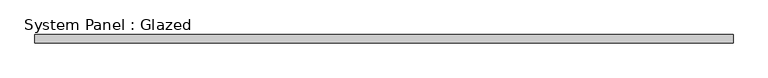
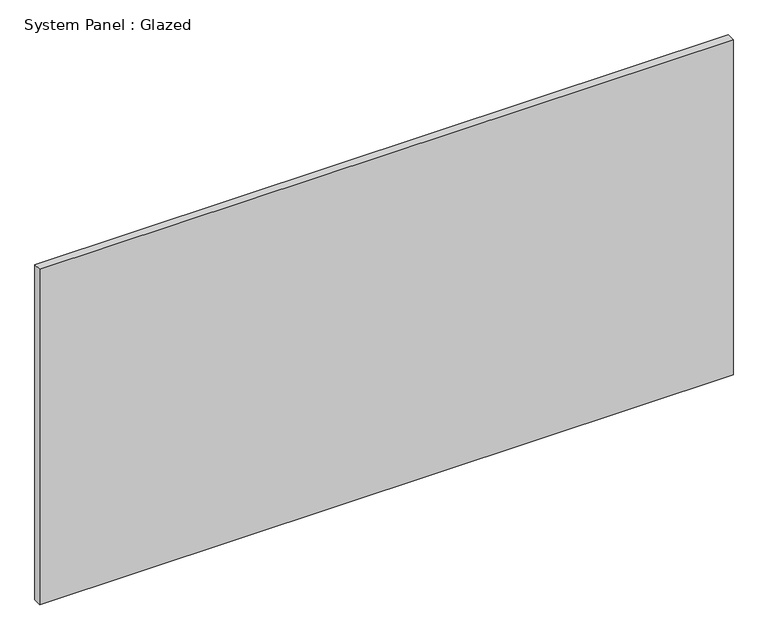
"""IFC4 building model written with IfcOpenShell, lengths in millimetres: plate geometry, System Panel : Glazed."""

from ifc_helpers import new_model, si_unit, origin, origin_with_axes, place, context, project, spatial, polyline, outline, extrude, source, transform, mapped, element, save


def system_panel_glazed_5a0db22b(model_context):
    return source(origin(), model_context, "Body", "SweptSolid", [
        extrude(outline(polyline([(1079.5, 19.05), (-1079.5, 19.05), (-1079.5, 44.45), (1079.5, 44.45), (1079.5, 19.05)])), origin_with_axes(), (0.0, 0.0, 1.0), 1103.8821304),
    ])


if __name__ == "__main__":
    model = new_model("IFC4")
    model_context = context("Model", 3, world=origin())
    ifc_project = project(units=[si_unit("LENGTHUNIT", "METRE", prefix="MILLI")], contexts=[model_context])
    site = spatial("IfcSite", under=ifc_project)
    building = spatial("IfcBuilding", under=site)
    placement = place(None, origin())
    system_panel_glazed_shape = system_panel_glazed_5a0db22b(model_context)
    element("IfcPlate", 1, ObjectType="System Panel : Glazed", at=placement, inside=building, context=model_context, shape_type="MappedRepresentation", body=[
        mapped(system_panel_glazed_shape, transform((0.0, 0.0, 0.0), x_axis=(1.0, 0.0, 0.0), y_axis=(0.0, 1.0, 0.0), z_axis=(0.0, 0.0, 1.0))),
    ])
    save(model, "model.ifc")

# Revit data of these elements
# Type "System Panel : Glazed"
#   Construction Type Id = "GSP4R"
#   Analytic Construction = "1/8 in Pilkington single glazing"
#   Visual Light Transmittance = 0.9
#   Solar Heat Gain Coefficient = 0.86
#   Heat Transfer Coefficient (U) = 1.18115 BTU/(h·ft²·°F)
# Element 1 (IfcPlate, "System Panel : Glazed")
#   Materials on its faces: "Glass"
# Materials
#   "Glass": class "Glass", colour RGB 0 128 192, transparency 0.75, Description = "Soda Lime Glass", Cost = 0
